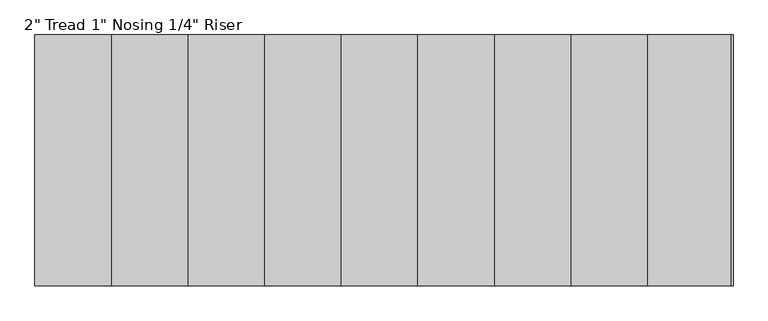
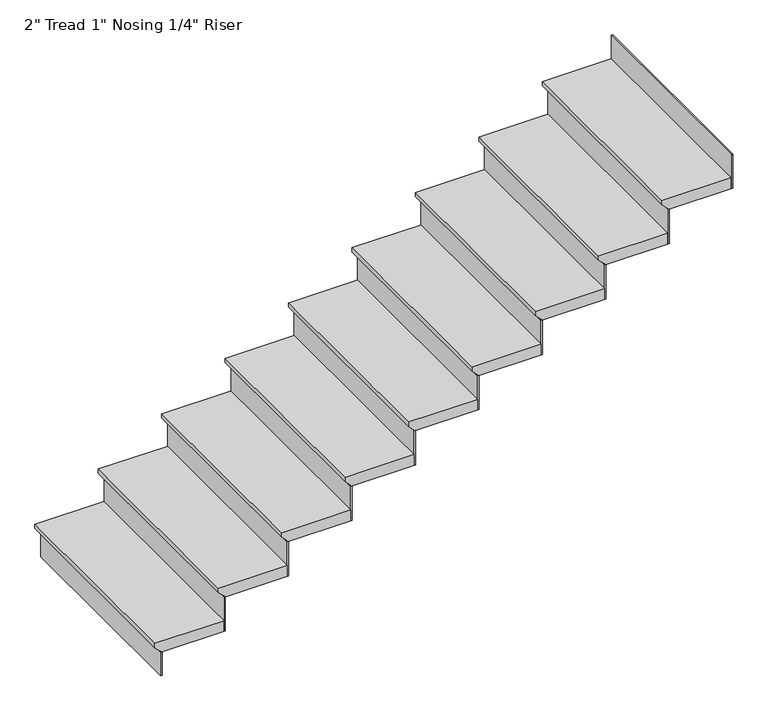
"""IFC4 building model written with IfcOpenShell, lengths in millimetres: stair flight geometry."""

from ifc_helpers import new_model, si_unit, origin, place, context, project, spatial, faceted_brep, source, transform, mapped, element, save


def stair_flight_e0f3031c(model_context):
    return source(origin(), model_context, "Body", "Brep", [
        faceted_brep([(-1591.1154463, -4737.3544725, 19343.37), (-1591.1154463, -4737.3544725, 19362.42), (-1591.1154463, -3822.9544725, 19362.42), (-1591.1154463, -3822.9544725, 19343.37), (-1565.7154463, -4737.3544725, 19317.97), (-1565.7154463, -3822.9544725, 19317.97), (-1286.3154463, -4737.3544725, 19362.42), (-1286.3154463, -3822.9544725, 19362.42), (-1565.7154463, -3822.9544725, 19311.62), (-1286.3154463, -3822.9544725, 19311.62), (-1286.3154463, -4737.3544725, 19311.62), (-1565.7154463, -4737.3544725, 19311.62)], [[[0, 1, 2, 3]], [[4, 0, 3, 5]], [[2, 1, 6, 7]], [[8, 9, 10, 11]], [[2, 7, 9, 8, 5, 3]], [[8, 11, 4, 5]], [[6, 1, 0, 4, 11, 10]], [[7, 6, 10, 9]]]),
        faceted_brep([(-1565.7154463, -4737.3544725, 19311.62), (-1565.7154463, -4737.3544725, 19202.4), (-1559.3654463, -4737.3544725, 19202.4), (-1559.3654463, -4737.3544725, 19311.62), (-1565.7154463, -3822.9544725, 19311.62), (-1559.3654463, -3822.9544725, 19311.62), (-1559.3654463, -3822.9544725, 19202.4), (-1565.7154463, -3822.9544725, 19202.4)], [[[0, 1, 2, 3]], [[4, 5, 6, 7]], [[1, 0, 4, 7]], [[2, 1, 7, 6]], [[3, 2, 6, 5]], [[0, 3, 5, 4]]]),
        faceted_brep([(-1286.3154463, -4737.3544725, 19471.64), (-1286.3154463, -4737.3544725, 19311.62), (-1279.9654463, -4737.3544725, 19311.62), (-1279.9654463, -4737.3544725, 19471.64), (-1286.3154463, -3822.9544725, 19471.64), (-1279.9654463, -3822.9544725, 19471.64), (-1279.9654463, -3822.9544725, 19311.62), (-1286.3154463, -3822.9544725, 19311.62)], [[[0, 1, 2, 3]], [[4, 5, 6, 7]], [[1, 0, 4, 7]], [[2, 1, 7, 6]], [[3, 2, 6, 5]], [[0, 3, 5, 4]]]),
        faceted_brep([(-1311.7154463, -3822.9544725, 19522.44), (-1311.7154463, -4737.3544725, 19522.44), (-1006.9154463, -4737.3544725, 19522.44), (-1006.9154463, -3822.9544725, 19522.44), (-1286.3154463, -3822.9544725, 19471.64), (-1006.9154463, -3822.9544725, 19471.64), (-1006.9154463, -4737.3544725, 19471.64), (-1286.3154463, -4737.3544725, 19471.64), (-1286.3154463, -3822.9544725, 19477.99), (-1311.7154463, -3822.9544725, 19503.39), (-1286.3154463, -4737.3544725, 19477.99), (-1311.7154463, -4737.3544725, 19503.39)], [[[0, 1, 2, 3]], [[4, 5, 6, 7]], [[0, 3, 5, 4, 8, 9]], [[4, 7, 10, 8]], [[2, 1, 11, 10, 7, 6]], [[3, 2, 6, 5]], [[11, 1, 0, 9]], [[10, 11, 9, 8]]]),
        faceted_brep([(-1006.9154463, -4737.3544725, 19631.66), (-1006.9154463, -4737.3544725, 19471.64), (-1000.5654463, -4737.3544725, 19471.64), (-1000.5654463, -4737.3544725, 19631.66), (-1006.9154463, -3822.9544725, 19631.66), (-1000.5654463, -3822.9544725, 19631.66), (-1000.5654463, -3822.9544725, 19471.64), (-1006.9154463, -3822.9544725, 19471.64)], [[[0, 1, 2, 3]], [[4, 5, 6, 7]], [[1, 0, 4, 7]], [[2, 1, 7, 6]], [[3, 2, 6, 5]], [[0, 3, 5, 4]]]),
        faceted_brep([(-1032.3154463, -3822.9544725, 19682.46), (-1032.3154463, -4737.3544725, 19682.46), (-727.5154463, -4737.3544725, 19682.46), (-727.5154463, -3822.9544725, 19682.46), (-1006.9154463, -3822.9544725, 19631.66), (-727.5154463, -3822.9544725, 19631.66), (-727.5154463, -4737.3544725, 19631.66), (-1006.9154463, -4737.3544725, 19631.66), (-1006.9154463, -3822.9544725, 19638.01), (-1032.3154463, -3822.9544725, 19663.41), (-1006.9154463, -4737.3544725, 19638.01), (-1032.3154463, -4737.3544725, 19663.41)], [[[0, 1, 2, 3]], [[4, 5, 6, 7]], [[0, 3, 5, 4, 8, 9]], [[4, 7, 10, 8]], [[2, 1, 11, 10, 7, 6]], [[3, 2, 6, 5]], [[11, 1, 0, 9]], [[10, 11, 9, 8]]]),
        faceted_brep([(-727.5154463, -4737.3544725, 19791.68), (-727.5154463, -4737.3544725, 19631.66), (-721.1654463, -4737.3544725, 19631.66), (-721.1654463, -4737.3544725, 19791.68), (-727.5154463, -3822.9544725, 19791.68), (-721.1654463, -3822.9544725, 19791.68), (-721.1654463, -3822.9544725, 19631.66), (-727.5154463, -3822.9544725, 19631.66)], [[[0, 1, 2, 3]], [[4, 5, 6, 7]], [[1, 0, 4, 7]], [[2, 1, 7, 6]], [[3, 2, 6, 5]], [[0, 3, 5, 4]]]),
        faceted_brep([(-752.9154463, -3822.9544725, 19842.48), (-752.9154463, -4737.3544725, 19842.48), (-448.1154463, -4737.3544725, 19842.48), (-448.1154463, -3822.9544725, 19842.48), (-727.5154463, -3822.9544725, 19791.68), (-448.1154463, -3822.9544725, 19791.68), (-448.1154463, -4737.3544725, 19791.68), (-727.5154463, -4737.3544725, 19791.68), (-727.5154463, -3822.9544725, 19798.03), (-752.9154463, -3822.9544725, 19823.43), (-727.5154463, -4737.3544725, 19798.03), (-752.9154463, -4737.3544725, 19823.43)], [[[0, 1, 2, 3]], [[4, 5, 6, 7]], [[0, 3, 5, 4, 8, 9]], [[4, 7, 10, 8]], [[2, 1, 11, 10, 7, 6]], [[3, 2, 6, 5]], [[11, 1, 0, 9]], [[10, 11, 9, 8]]]),
        faceted_brep([(-448.1154463, -4737.3544725, 19951.7), (-448.1154463, -4737.3544725, 19791.68), (-441.7654463, -4737.3544725, 19791.68), (-441.7654463, -4737.3544725, 19951.7), (-448.1154463, -3822.9544725, 19951.7), (-441.7654463, -3822.9544725, 19951.7), (-441.7654463, -3822.9544725, 19791.68), (-448.1154463, -3822.9544725, 19791.68)], [[[0, 1, 2, 3]], [[4, 5, 6, 7]], [[1, 0, 4, 7]], [[2, 1, 7, 6]], [[3, 2, 6, 5]], [[0, 3, 5, 4]]]),
        faceted_brep([(-473.5154463, -3822.9544725, 20002.5), (-473.5154463, -4737.3544725, 20002.5), (-168.7154463, -4737.3544725, 20002.5), (-168.7154463, -3822.9544725, 20002.5), (-448.1154463, -3822.9544725, 19951.7), (-168.7154463, -3822.9544725, 19951.7), (-168.7154463, -4737.3544725, 19951.7), (-448.1154463, -4737.3544725, 19951.7), (-448.1154463, -3822.9544725, 19958.05), (-473.5154463, -3822.9544725, 19983.45), (-448.1154463, -4737.3544725, 19958.05), (-473.5154463, -4737.3544725, 19983.45)], [[[0, 1, 2, 3]], [[4, 5, 6, 7]], [[0, 3, 5, 4, 8, 9]], [[4, 7, 10, 8]], [[2, 1, 11, 10, 7, 6]], [[3, 2, 6, 5]], [[11, 1, 0, 9]], [[10, 11, 9, 8]]]),
        faceted_brep([(-168.7154463, -4737.3544725, 20111.72), (-168.7154463, -4737.3544725, 19951.7), (-162.3654463, -4737.3544725, 19951.7), (-162.3654463, -4737.3544725, 20111.72), (-168.7154463, -3822.9544725, 20111.72), (-162.3654463, -3822.9544725, 20111.72), (-162.3654463, -3822.9544725, 19951.7), (-168.7154463, -3822.9544725, 19951.7)], [[[0, 1, 2, 3]], [[4, 5, 6, 7]], [[1, 0, 4, 7]], [[2, 1, 7, 6]], [[3, 2, 6, 5]], [[0, 3, 5, 4]]]),
        faceted_brep([(-194.1154463, -3822.9544725, 20162.52), (-194.1154463, -4737.3544725, 20162.52), (110.6845537, -4737.3544725, 20162.52), (110.6845537, -3822.9544725, 20162.52), (-168.7154463, -3822.9544725, 20111.72), (110.6845537, -3822.9544725, 20111.72), (110.6845537, -4737.3544725, 20111.72), (-168.7154463, -4737.3544725, 20111.72), (-168.7154463, -3822.9544725, 20118.07), (-194.1154463, -3822.9544725, 20143.47), (-168.7154463, -4737.3544725, 20118.07), (-194.1154463, -4737.3544725, 20143.47)], [[[0, 1, 2, 3]], [[4, 5, 6, 7]], [[0, 3, 5, 4, 8, 9]], [[4, 7, 10, 8]], [[2, 1, 11, 10, 7, 6]], [[3, 2, 6, 5]], [[11, 1, 0, 9]], [[10, 11, 9, 8]]]),
        faceted_brep([(110.6845537, -4737.3544725, 20271.74), (110.6845537, -4737.3544725, 20111.72), (117.0345537, -4737.3544725, 20111.72), (117.0345537, -4737.3544725, 20271.74), (110.6845537, -3822.9544725, 20271.74), (117.0345537, -3822.9544725, 20271.74), (117.0345537, -3822.9544725, 20111.72), (110.6845537, -3822.9544725, 20111.72)], [[[0, 1, 2, 3]], [[4, 5, 6, 7]], [[1, 0, 4, 7]], [[2, 1, 7, 6]], [[3, 2, 6, 5]], [[0, 3, 5, 4]]]),
        faceted_brep([(85.2845537, -3822.9544725, 20322.54), (85.2845537, -4737.3544725, 20322.54), (390.0845537, -4737.3544725, 20322.54), (390.0845537, -3822.9544725, 20322.54), (110.6845537, -3822.9544725, 20271.74), (390.0845537, -3822.9544725, 20271.74), (390.0845537, -4737.3544725, 20271.74), (110.6845537, -4737.3544725, 20271.74), (110.6845537, -3822.9544725, 20278.09), (85.2845537, -3822.9544725, 20303.49), (110.6845537, -4737.3544725, 20278.09), (85.2845537, -4737.3544725, 20303.49)], [[[0, 1, 2, 3]], [[4, 5, 6, 7]], [[0, 3, 5, 4, 8, 9]], [[4, 7, 10, 8]], [[2, 1, 11, 10, 7, 6]], [[3, 2, 6, 5]], [[11, 1, 0, 9]], [[10, 11, 9, 8]]]),
        faceted_brep([(390.0845537, -4737.3544725, 20431.76), (390.0845537, -4737.3544725, 20271.74), (396.4345537, -4737.3544725, 20271.74), (396.4345537, -4737.3544725, 20431.76), (390.0845537, -3822.9544725, 20431.76), (396.4345537, -3822.9544725, 20431.76), (396.4345537, -3822.9544725, 20271.74), (390.0845537, -3822.9544725, 20271.74)], [[[0, 1, 2, 3]], [[4, 5, 6, 7]], [[1, 0, 4, 7]], [[2, 1, 7, 6]], [[3, 2, 6, 5]], [[0, 3, 5, 4]]]),
        faceted_brep([(364.6845537, -3822.9544725, 20482.56), (364.6845537, -4737.3544725, 20482.56), (669.4845537, -4737.3544725, 20482.56), (669.4845537, -3822.9544725, 20482.56), (390.0845537, -3822.9544725, 20431.76), (669.4845537, -3822.9544725, 20431.76), (669.4845537, -4737.3544725, 20431.76), (390.0845537, -4737.3544725, 20431.76), (390.0845537, -3822.9544725, 20438.11), (364.6845537, -3822.9544725, 20463.51), (390.0845537, -4737.3544725, 20438.11), (364.6845537, -4737.3544725, 20463.51)], [[[0, 1, 2, 3]], [[4, 5, 6, 7]], [[0, 3, 5, 4, 8, 9]], [[4, 7, 10, 8]], [[2, 1, 11, 10, 7, 6]], [[3, 2, 6, 5]], [[11, 1, 0, 9]], [[10, 11, 9, 8]]]),
        faceted_brep([(948.8845537, -4737.3544725, 20751.8), (948.8845537, -4737.3544725, 20591.78), (955.2345537, -4737.3544725, 20591.78), (955.2345537, -4737.3544725, 20751.8), (948.8845537, -3822.9544725, 20751.8), (955.2345537, -3822.9544725, 20751.8), (955.2345537, -3822.9544725, 20591.78), (948.8845537, -3822.9544725, 20591.78)], [[[0, 1, 2, 3]], [[4, 5, 6, 7]], [[1, 0, 4, 7]], [[2, 1, 7, 6]], [[3, 2, 6, 5]], [[0, 3, 5, 4]]]),
        faceted_brep([(669.4845537, -4737.3544725, 20591.78), (669.4845537, -4737.3544725, 20431.76), (675.8345537, -4737.3544725, 20431.76), (675.8345537, -4737.3544725, 20591.78), (669.4845537, -3822.9544725, 20591.78), (675.8345537, -3822.9544725, 20591.78), (675.8345537, -3822.9544725, 20431.76), (669.4845537, -3822.9544725, 20431.76)], [[[0, 1, 2, 3]], [[4, 5, 6, 7]], [[1, 0, 4, 7]], [[2, 1, 7, 6]], [[3, 2, 6, 5]], [[0, 3, 5, 4]]]),
        faceted_brep([(948.8845537, -3822.9544725, 20642.58), (923.4845537, -3822.9544725, 20642.58), (644.0845537, -3822.9544725, 20642.58), (644.0845537, -4737.3544725, 20642.58), (948.8845537, -4737.3544725, 20642.58), (923.4845537, -3822.9544725, 20591.78), (948.8845537, -3822.9544725, 20591.78), (948.8845537, -4737.3544725, 20591.78), (669.4845537, -4737.3544725, 20591.78), (669.4845537, -3822.9544725, 20591.78), (669.4845537, -3822.9544725, 20598.13), (644.0845537, -3822.9544725, 20623.53), (669.4845537, -4737.3544725, 20598.13), (644.0845537, -4737.3544725, 20623.53)], [[[0, 1, 2, 3, 4]], [[5, 6, 7, 8, 9]], [[1, 0, 6, 5]], [[2, 1, 5, 9, 10, 11]], [[9, 8, 12, 10]], [[4, 3, 13, 12, 8, 7]], [[0, 4, 7, 6]], [[13, 3, 2, 11]], [[12, 13, 11, 10]]]),
    ])


if __name__ == "__main__":
    model = new_model("IFC4")
    model_context = context("Model", 3, world=origin())
    ifc_project = project(units=[si_unit("LENGTHUNIT", "METRE", prefix="MILLI")], contexts=[model_context])
    site = spatial("IfcSite", under=ifc_project)
    building = spatial("IfcBuilding", under=site)
    placement = place(None, origin())
    stair_flight_shape = stair_flight_e0f3031c(model_context)
    element("IfcStairFlight", 1, ObjectType="2\" Tread 1\" Nosing 1/4\" Riser", at=placement, inside=building, context=model_context, shape_type="MappedRepresentation", body=[
        mapped(stair_flight_shape, transform((0.0, 0.0, 0.0), x_axis=(1.0, 0.0, 0.0), y_axis=(0.0, 1.0, 0.0), z_axis=(0.0, 0.0, 1.0))),
    ])
    save(model, "model.ifc")
